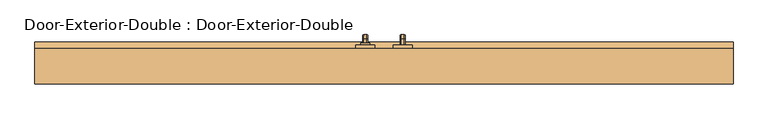
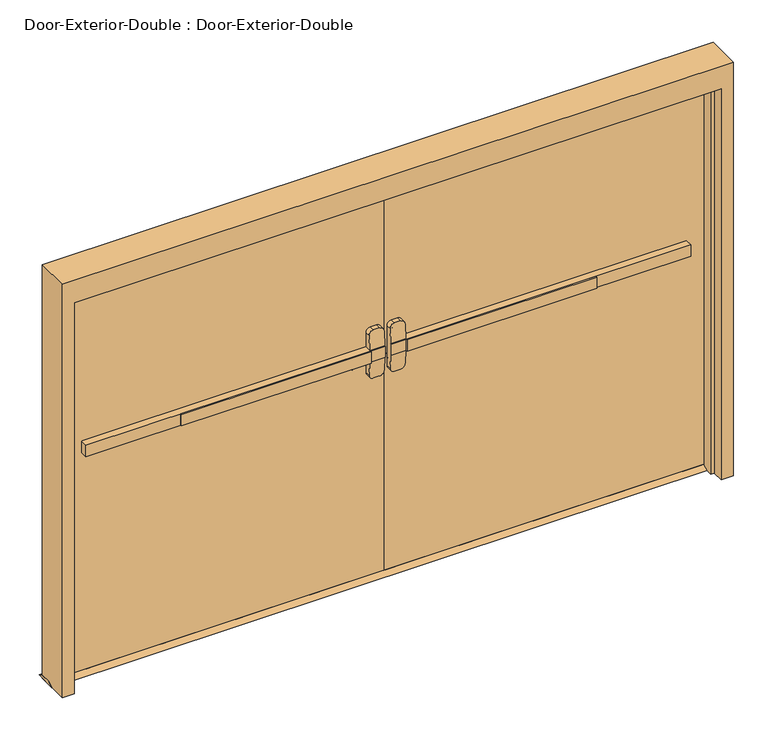
"""IFC4 building model written with IfcOpenShell, lengths in millimetres: door geometry, Door-Exterior-Double : Door-Exterior-Double."""

from ifc_helpers import new_model, si_unit, point, frame, frame_2d, origin, place, context, project, spatial, polyline, circle_curve, ellipse_curve, trimmed, segment, composite_curve, outline, extrude, faceted_brep, source, transform, mapped, element, save
from ifc_brep_helpers import plane_surface, cylinder_surface, revolved_surface, advanced_brep


def door_exterior_double_door_exterior_double_ceddc7a2(model_context):
    return source(origin(), model_context, "Body", "SolidModel", [
        extrude(outline(polyline([(-880.5333333, 0.0), (-880.5333333, 6.35), (-76.2, 6.35), (-76.2, 0.0), (-880.5333333, 0.0)])), frame((0.0, 0.0, 990.6), z_axis=(0.0, 0.0, 1.0), x_axis=(1.0, 0.0, 0.0)), (0.0, 0.0, 1.0), 50.8),
        advanced_brep(
        [(-12.7, 6.35, 1041.4), (-76.2, 6.35, 1041.4), (-1282.7, 6.35, 1041.4), (-1282.7, 6.35, 990.6), (-76.2, 6.35, 990.6), (-12.7, 6.35, 990.6), (-1282.7, 38.1, 1041.4), (-76.2, 38.1, 1041.4), (-76.2, 38.1, 1104.9), (-57.15, 38.1, 1123.95), (-31.75, 38.1, 1123.95), (-12.7, 38.1, 1104.9), (-12.7, 38.1, 927.1), (-31.75, 38.1, 908.05), (-57.15, 38.1, 908.05), (-76.2, 38.1, 927.1), (-76.2, 38.1, 990.6), (-1282.7, 38.1, 990.6), (-12.7, 9.5252467, 1041.4), (-76.2, 9.5252467, 1041.4), (-12.7, 9.5252467, 990.6), (-12.7, 14.5354269, 927.1), (-12.7, 14.5354269, 1104.9), (-76.2, 9.5252467, 990.6), (-76.2, 14.5354269, 1104.9), (-76.2, 14.5354269, 927.1), (-57.15, 16.038481, 1123.95), (-31.75, 16.038481, 1123.95), (-31.75, 16.038481, 908.05), (-57.15, 16.038481, 908.05)],
        [
            (0, 1),
            (1, 2),
            (2, 3),
            (3, 4),
            (4, 5),
            (5, 0),
            (6, 7),
            (7, 8),
            (8, 9, circle_curve(frame((-57.15, 38.1, 1104.9), z_axis=(0.0, 1.0, 0.0), x_axis=(-1.0, 0.0, 0.0)), 19.05)),
            (9, 10),
            (10, 11, circle_curve(frame((-31.75, 38.1, 1104.9), z_axis=(0.0, 1.0, 0.0), x_axis=(-1.0, 0.0, 0.0)), 19.05)),
            (11, 12),
            (12, 13, circle_curve(frame((-31.75, 38.1, 927.1), z_axis=(0.0, 1.0, 0.0), x_axis=(-1.0, 0.0, 0.0)), 19.05)),
            (13, 14),
            (14, 15, circle_curve(frame((-57.15, 38.1, 927.1), z_axis=(0.0, 1.0, 0.0), x_axis=(-1.0, 0.0, 0.0)), 19.05)),
            (15, 16),
            (16, 17),
            (17, 6),
            (0, 18),
            (18, 19),
            (19, 7),
            (6, 2),
            (5, 20),
            (20, 21),
            (21, 12),
            (11, 22),
            (22, 18),
            (16, 23),
            (23, 20),
            (3, 17),
            (19, 24),
            (24, 8),
            (15, 25),
            (25, 23),
            (9, 26),
            (26, 27),
            (27, 10),
            (13, 28),
            (28, 29),
            (29, 14),
            (29, 25, ellipse_curve(frame((-57.15, 14.5354269, 927.1), z_axis=(0.0, 0.9969018152893365, 0.07865602756830282), x_axis=(0.0, -0.07865602756830208, 0.9969018152893365)), 19.1092038, 19.05)),
            (24, 26, ellipse_curve(frame((-57.15, 14.5354269, 1104.9), z_axis=(0.0, 0.9969018152893376, -0.07865602756828934), x_axis=(0.0, -0.078656027568288, -0.9969018152893377)), 19.1092038, 19.05)),
            (27, 22, ellipse_curve(frame((-31.75, 14.5354269, 1104.9), z_axis=(0.0, 0.9969018152893376, -0.07865602756828934), x_axis=(0.0, -0.078656027568288, -0.9969018152893377)), 19.1092038, 19.05)),
            (21, 28, ellipse_curve(frame((-31.75, 14.5354269, 927.1), z_axis=(0.0, 0.9969018152893365, 0.07865602756830282), x_axis=(0.0, -0.07865602756830208, 0.9969018152893365)), 19.1092038, 19.05)),
        ],
        [
            plane_surface(frame((-12.7, 6.35, 1041.4), z_axis=(0.0, -1.0, 0.0), x_axis=(1.0, 0.0, 0.0))),
            plane_surface(frame((-12.7, 38.1, 1041.4), z_axis=(0.0, 1.0, 0.0), x_axis=(-1.0, 0.0, 0.0))),
            plane_surface(frame((-1282.7, 6.35, 1041.4), z_axis=(0.0, 0.0, 1.0), x_axis=(0.0, 1.0, 0.0))),
            plane_surface(frame((-12.7, 6.35, 1041.4), z_axis=(1.0, 0.0, 0.0), x_axis=(0.0, 1.0, 0.0))),
            plane_surface(frame((-12.7, 6.35, 990.6), z_axis=(0.0, 0.0, -1.0), x_axis=(0.0, 1.0, 0.0))),
            plane_surface(frame((-1282.7, 6.35, 990.6), z_axis=(-1.0, 0.0, 0.0), x_axis=(0.0, 1.0, 0.0))),
            plane_surface(frame((-76.2, 9.5252467, 927.1), z_axis=(-1.0, 0.0, 0.0), x_axis=(0.0, 1.0, 0.0))),
            plane_surface(frame((-57.15, 9.5252467, 1123.95), z_axis=(0.0, 0.0, 1.0), x_axis=(0.0, 1.0, 0.0))),
            plane_surface(frame((-31.75, 9.5252467, 908.05), z_axis=(0.0, 0.0, -1.0), x_axis=(0.0, 1.0, 0.0))),
            cylinder_surface(frame((-57.15, 38.1, 927.1), z_axis=(0.0, -1.0, 0.0), x_axis=(-1.0, 0.0, 0.0)), 19.05),
            cylinder_surface(frame((-57.15, 38.1, 1104.9), z_axis=(0.0, -1.0, 0.0), x_axis=(-1.0, 0.0, 0.0)), 19.05),
            cylinder_surface(frame((-31.75, 38.1, 1104.9), z_axis=(0.0, -1.0, 0.0), x_axis=(-1.0, 0.0, 0.0)), 19.05),
            cylinder_surface(frame((-31.75, 38.1, 927.1), z_axis=(0.0, -1.0, 0.0), x_axis=(-1.0, 0.0, 0.0)), 19.05),
            plane_surface(frame((-76.2, 9.5252467, 1041.4), z_axis=(0.0, -0.9969018152893376, 0.07865602756828934), x_axis=(1.0, 0.0, 0.0))),
            plane_surface(frame((-76.2, 16.038481, 908.05), z_axis=(0.0, -0.9969018152893365, -0.07865602756830282), x_axis=(1.0, 0.0, 0.0))),
        ],
        [
            (0, [[1, 2, 3, 4, 5, 6]]),
            (1, [[7, 8, 9, 10, 11, 12, 13, 14, 15, 16, 17, 18]]),
            (2, [[-2, -1, 19, 20, 21, -7, 22]]),
            (3, [[23, 24, 25, -12, 26, 27, -19, -6]]),
            (4, [[-17, 28, 29, -23, -5, -4, 30]]),
            (5, [[-22, -18, -30, -3]]),
            (6, [[-21, 31, 32, -8]]),
            (6, [[33, 34, -28, -16]]),
            (7, [[35, 36, 37, -10]]),
            (8, [[38, 39, 40, -14]]),
            (9, [[-40, 41, -33, -15]]),
            (10, [[-32, 42, -35, -9]]),
            (11, [[-37, 43, -26, -11]]),
            (12, [[-25, 44, -38, -13]]),
            (13, [[-27, -43, -36, -42, -31, -20]]),
            (14, [[-29, -34, -41, -39, -44, -24]]),
        ],
    ),
        extrude(outline(polyline([(82.55, 12.7), (107.95, 0.0), (12.7, 0.0), (38.1, 12.7), (82.55, 12.7)])), frame((-1422.4, 0.0, 0.0), z_axis=(1.0, 0.0, 0.0), x_axis=(0.0, 1.0, 0.0)), (0.0, 0.0, 1.0), 2844.8),
        extrude(outline(polyline([(880.5333333, 0.0), (76.2, 0.0), (76.2, 6.35), (880.5333333, 6.35), (880.5333333, 0.0)])), frame((0.0, 0.0, 990.6), z_axis=(0.0, 0.0, 1.0), x_axis=(1.0, 0.0, 0.0)), (0.0, 0.0, 1.0), 50.8),
        advanced_brep(
        [(12.7, 6.35, 1041.4), (12.7, 6.35, 990.6), (76.2, 6.35, 990.6), (1282.7, 6.35, 990.6), (1282.7, 6.35, 1041.4), (76.2, 6.35, 1041.4), (1282.7, 38.1, 1041.4), (1282.7, 38.1, 990.6), (76.2, 38.1, 990.6), (76.2, 38.1, 927.1), (57.15, 38.1, 908.05), (31.75, 38.1, 908.05), (12.7, 38.1, 927.1), (12.7, 38.1, 1104.9), (31.75, 38.1, 1123.95), (57.15, 38.1, 1123.95), (76.2, 38.1, 1104.9), (76.2, 38.1, 1041.4), (76.2, 9.5252467, 1041.4), (12.7, 9.5252467, 1041.4), (12.7, 14.5354269, 1104.9), (12.7, 14.5354269, 927.1), (12.7, 9.5252467, 990.6), (76.2, 9.5252467, 990.6), (76.2, 14.5354269, 927.1), (76.2, 14.5354269, 1104.9), (31.75, 16.038481, 1123.95), (57.15, 16.038481, 1123.95), (57.15, 16.038481, 908.05), (31.75, 16.038481, 908.05)],
        [
            (0, 1),
            (1, 2),
            (2, 3),
            (3, 4),
            (4, 5),
            (5, 0),
            (6, 7),
            (7, 8),
            (8, 9),
            (9, 10, circle_curve(frame((57.15, 38.1, 927.1), z_axis=(0.0, 1.0, 0.0), x_axis=(1.0, 0.0, 0.0)), 19.05)),
            (10, 11),
            (11, 12, circle_curve(frame((31.75, 38.1, 927.1), z_axis=(0.0, 1.0, 0.0), x_axis=(1.0, 0.0, 0.0)), 19.05)),
            (12, 13),
            (13, 14, circle_curve(frame((31.75, 38.1, 1104.9), z_axis=(0.0, 1.0, 0.0), x_axis=(1.0, 0.0, 0.0)), 19.05)),
            (14, 15),
            (15, 16, circle_curve(frame((57.15, 38.1, 1104.9), z_axis=(0.0, 1.0, 0.0), x_axis=(1.0, 0.0, 0.0)), 19.05)),
            (16, 17),
            (17, 6),
            (4, 6),
            (17, 18),
            (18, 19),
            (19, 0),
            (19, 20),
            (20, 13),
            (12, 21),
            (21, 22),
            (22, 1),
            (7, 3),
            (22, 23),
            (23, 8),
            (23, 24),
            (24, 9),
            (16, 25),
            (25, 18),
            (14, 26),
            (26, 27),
            (27, 15),
            (10, 28),
            (28, 29),
            (29, 11),
            (24, 28, ellipse_curve(frame((57.15, 14.5354269, 927.1), z_axis=(0.0, 0.9969018152893365, 0.07865602756830282), x_axis=(0.0, -0.07865602756830208, 0.9969018152893365)), 19.1092038, 19.05)),
            (27, 25, ellipse_curve(frame((57.15, 14.5354269, 1104.9), z_axis=(0.0, 0.9969018152893376, -0.07865602756828934), x_axis=(0.0, -0.078656027568288, -0.9969018152893377)), 19.1092038, 19.05)),
            (20, 26, ellipse_curve(frame((31.75, 14.5354269, 1104.9), z_axis=(0.0, 0.9969018152893376, -0.07865602756828934), x_axis=(0.0, -0.078656027568288, -0.9969018152893377)), 19.1092038, 19.05)),
            (29, 21, ellipse_curve(frame((31.75, 14.5354269, 927.1), z_axis=(0.0, 0.9969018152893365, 0.07865602756830282), x_axis=(0.0, -0.07865602756830208, 0.9969018152893365)), 19.1092038, 19.05)),
        ],
        [
            plane_surface(frame((12.7, 6.35, 1041.4), z_axis=(0.0, -1.0, 0.0), x_axis=(-1.0, 0.0, 0.0))),
            plane_surface(frame((12.7, 38.1, 1041.4), z_axis=(0.0, 1.0, 0.0), x_axis=(1.0, 0.0, 0.0))),
            plane_surface(frame((1282.7, 6.35, 1041.4), z_axis=(0.0, 0.0, 1.0), x_axis=(0.0, 1.0, 0.0))),
            plane_surface(frame((12.7, 6.35, 1041.4), z_axis=(-1.0, 0.0, 0.0), x_axis=(0.0, 1.0, 0.0))),
            plane_surface(frame((12.7, 6.35, 990.6), z_axis=(0.0, 0.0, -1.0), x_axis=(0.0, 1.0, 0.0))),
            plane_surface(frame((1282.7, 6.35, 990.6), z_axis=(1.0, 0.0, 0.0), x_axis=(0.0, 1.0, 0.0))),
            plane_surface(frame((76.2, 9.5252467, 927.1), z_axis=(1.0, 0.0, 0.0), x_axis=(0.0, 1.0, 0.0))),
            plane_surface(frame((57.15, 9.5252467, 1123.95), z_axis=(0.0, 0.0, 1.0), x_axis=(0.0, 1.0, 0.0))),
            plane_surface(frame((31.75, 9.5252467, 908.05), z_axis=(0.0, 0.0, -1.0), x_axis=(0.0, 1.0, 0.0))),
            cylinder_surface(frame((57.15, 38.1, 927.1), z_axis=(0.0, -1.0, 0.0), x_axis=(1.0, 0.0, 0.0)), 19.05),
            cylinder_surface(frame((57.15, 38.1, 1104.9), z_axis=(0.0, -1.0, 0.0), x_axis=(1.0, 0.0, 0.0)), 19.05),
            cylinder_surface(frame((31.75, 38.1, 1104.9), z_axis=(0.0, -1.0, 0.0), x_axis=(1.0, 0.0, 0.0)), 19.05),
            cylinder_surface(frame((31.75, 38.1, 927.1), z_axis=(0.0, -1.0, 0.0), x_axis=(1.0, 0.0, 0.0)), 19.05),
            plane_surface(frame((76.2, 9.5252467, 1041.4), z_axis=(0.0, -0.9969018152893376, 0.07865602756828934), x_axis=(-1.0, 0.0, 0.0))),
            plane_surface(frame((76.2, 16.038481, 908.05), z_axis=(0.0, -0.9969018152893365, -0.07865602756830282), x_axis=(-1.0, 0.0, 0.0))),
        ],
        [
            (0, [[1, 2, 3, 4, 5, 6]]),
            (1, [[7, 8, 9, 10, 11, 12, 13, 14, 15, 16, 17, 18]]),
            (2, [[19, -18, 20, 21, 22, -6, -5]]),
            (3, [[-1, -22, 23, 24, -13, 25, 26, 27]]),
            (4, [[28, -3, -2, -27, 29, 30, -8]]),
            (5, [[-4, -28, -7, -19]]),
            (6, [[-9, -30, 31, 32]]),
            (6, [[-17, 33, 34, -20]]),
            (7, [[-15, 35, 36, 37]]),
            (8, [[-11, 38, 39, 40]]),
            (9, [[-10, -32, 41, -38]]),
            (10, [[-16, -37, 42, -33]]),
            (11, [[-14, -24, 43, -35]]),
            (12, [[-12, -40, 44, -25]]),
            (13, [[-21, -34, -42, -36, -43, -23]]),
            (14, [[-26, -44, -39, -41, -31, -29]]),
        ],
    ),
        advanced_brep(
        [(66.2, 95.25, 1017.190625), (66.2, 95.25, 1014.809375), (69.771875, 95.25, 1011.2375), (82.6284594, 95.25, 1011.2375), (86.2, 95.25, 1014.8090406), (86.2, 95.25, 1017.190625), (82.628125, 95.25, 1020.7625), (69.771875, 95.25, 1020.7625), (66.2, 95.25, 887.809375), (69.771875, 95.25, 884.2375), (82.628125, 95.25, 884.2375), (86.2, 95.25, 887.809375), (86.2, 95.25, 890.1909594), (82.6284594, 95.25, 893.7625), (69.771875, 95.25, 893.7625), (66.2, 95.25, 890.190625), (66.2, 120.65, 1017.190625), (66.2, 134.540625, 1003.3), (66.2, 134.540625, 901.7), (66.2, 120.65, 887.809375), (66.2, 120.65, 890.190625), (66.2, 132.159375, 901.7), (66.2, 132.159375, 1003.3), (66.2, 120.65, 1014.809375), (69.771875, 120.65, 1011.2375), (82.6284594, 120.65, 1011.2375), (86.2, 120.65, 1014.8090406), (86.2, 132.1590406, 1003.3), (86.2, 132.1590406, 901.7), (86.2, 120.65, 890.1909594), (86.2, 120.65, 887.809375), (86.2, 134.540625, 901.7), (86.2, 134.540625, 1003.3), (86.2, 120.65, 1017.190625), (82.628125, 120.65, 1020.7625), (69.771875, 120.65, 1020.7625), (69.771875, 128.5875, 1003.3), (82.6284594, 128.5875, 1003.3), (82.628125, 138.1125, 1003.3), (69.771875, 138.1125, 1003.3), (69.771875, 128.5875, 901.7), (82.6284594, 128.5875, 901.7), (82.628125, 138.1125, 901.7), (69.771875, 138.1125, 901.7), (69.771875, 120.65, 893.7625), (82.6284594, 120.65, 893.7625), (82.628125, 120.65, 884.2375), (69.771875, 120.65, 884.2375)],
        [
            (0, 1),
            (1, 2, circle_curve(frame((69.771875, 95.25, 1014.809375), z_axis=(0.0, -1.0, 0.0), x_axis=(0.0, 0.0, 1.0)), 3.571875)),
            (2, 3),
            (3, 4, circle_curve(frame((82.6284594, 95.25, 1014.8090406), z_axis=(0.0, -1.0, 0.0), x_axis=(0.0, 0.0, 1.0)), 3.5715406)),
            (4, 5),
            (5, 6, circle_curve(frame((82.628125, 95.25, 1017.190625), z_axis=(0.0, -1.0, 0.0), x_axis=(0.0, 0.0, 1.0)), 3.571875)),
            (6, 7),
            (7, 0, circle_curve(frame((69.771875, 95.25, 1017.190625), z_axis=(0.0, -1.0, 0.0), x_axis=(0.0, 0.0, 1.0)), 3.571875)),
            (8, 9, circle_curve(frame((69.771875, 95.25, 887.809375), z_axis=(0.0, -1.0, 0.0), x_axis=(0.0, 0.0, -1.0)), 3.571875)),
            (9, 10),
            (10, 11, circle_curve(frame((82.628125, 95.25, 887.809375), z_axis=(0.0, -1.0, 0.0), x_axis=(0.0, 0.0, -1.0)), 3.571875)),
            (11, 12),
            (12, 13, circle_curve(frame((82.6284594, 95.25, 890.1909594), z_axis=(0.0, -1.0, 0.0), x_axis=(0.0, 0.0, -1.0)), 3.5715406)),
            (13, 14),
            (14, 15, circle_curve(frame((69.771875, 95.25, 890.190625), z_axis=(0.0, -1.0, 0.0), x_axis=(0.0, 0.0, -1.0)), 3.571875)),
            (15, 8),
            (0, 16),
            (16, 17, circle_curve(frame((66.2, 120.65, 1003.3), z_axis=(-1.0, 0.0, 0.0), x_axis=(0.0, 0.0, 1.0)), 13.890625)),
            (17, 18),
            (18, 19, circle_curve(frame((66.2, 120.65, 901.7), z_axis=(-1.0, 0.0, 0.0), x_axis=(0.0, 1.0, 0.0)), 13.890625)),
            (19, 8),
            (15, 20),
            (20, 21, circle_curve(frame((66.2, 120.65, 901.7), z_axis=(1.0, 0.0, 0.0), x_axis=(0.0, 1.0, 0.0)), 11.509375)),
            (21, 22),
            (22, 23, circle_curve(frame((66.2, 120.65, 1003.3), z_axis=(1.0, 0.0, 0.0), x_axis=(0.0, 0.0, 1.0)), 11.509375)),
            (23, 1),
            (23, 24, circle_curve(frame((69.771875, 120.65, 1014.809375), z_axis=(0.0, -1.0, 0.0), x_axis=(0.0, 0.0, 1.0)), 3.571875)),
            (24, 2),
            (24, 25),
            (25, 3),
            (25, 26, circle_curve(frame((82.6284594, 120.65, 1014.8090406), z_axis=(0.0, -1.0, 0.0), x_axis=(0.0, 0.0, 1.0)), 3.5715406)),
            (26, 4),
            (26, 27, circle_curve(frame((86.2, 120.65, 1003.3), z_axis=(-1.0, 0.0, 0.0), x_axis=(0.0, 0.0, 1.0)), 11.5090406)),
            (27, 28),
            (28, 29, circle_curve(frame((86.2, 120.65, 901.7), z_axis=(-1.0, 0.0, 0.0), x_axis=(0.0, 1.0, 0.0)), 11.5090406)),
            (29, 12),
            (11, 30),
            (30, 31, circle_curve(frame((86.2, 120.65, 901.7), z_axis=(1.0, 0.0, 0.0), x_axis=(0.0, 1.0, 0.0)), 13.890625)),
            (31, 32),
            (32, 33, circle_curve(frame((86.2, 120.65, 1003.3), z_axis=(1.0, 0.0, 0.0), x_axis=(0.0, 0.0, 1.0)), 13.890625)),
            (33, 5),
            (33, 34, circle_curve(frame((82.628125, 120.65, 1017.190625), z_axis=(0.0, -1.0, 0.0), x_axis=(0.0, 0.0, 1.0)), 3.571875)),
            (34, 6),
            (34, 35),
            (35, 7),
            (35, 16, circle_curve(frame((69.771875, 120.65, 1017.190625), z_axis=(0.0, -1.0, 0.0), x_axis=(0.0, 0.0, 1.0)), 3.571875)),
            (36, 24, circle_curve(frame((69.771875, 120.65, 1003.3), z_axis=(1.0, 0.0, 0.0), x_axis=(0.0, 0.0, 1.0)), 7.9375)),
            (22, 36, circle_curve(frame((69.771875, 132.159375, 1003.3), z_axis=(0.0, 0.0, 1.0), x_axis=(0.0, 1.0, 0.0)), 3.571875)),
            (37, 25, circle_curve(frame((82.6284594, 120.65, 1003.3), z_axis=(1.0, 0.0, 0.0), x_axis=(0.0, 0.0, 1.0)), 7.9375)),
            (36, 37),
            (37, 27, circle_curve(frame((82.6284594, 132.1590406, 1003.3), z_axis=(0.0, 0.0, 1.0), x_axis=(0.0, 1.0, 0.0)), 3.5715406)),
            (38, 34, circle_curve(frame((82.628125, 120.65, 1003.3), z_axis=(1.0, 0.0, 0.0), x_axis=(0.0, 0.0, 1.0)), 17.4625)),
            (32, 38, circle_curve(frame((82.628125, 134.540625, 1003.3), z_axis=(0.0, 0.0, 1.0), x_axis=(0.0, 1.0, 0.0)), 3.571875)),
            (39, 35, circle_curve(frame((69.771875, 120.65, 1003.3), z_axis=(1.0, 0.0, 0.0), x_axis=(0.0, 0.0, 1.0)), 17.4625)),
            (38, 39),
            (39, 17, circle_curve(frame((69.771875, 134.540625, 1003.3), z_axis=(0.0, 0.0, 1.0), x_axis=(0.0, 1.0, 0.0)), 3.571875)),
            (21, 40, circle_curve(frame((69.771875, 132.159375, 901.7), z_axis=(0.0, 0.0, 1.0), x_axis=(0.0, 1.0, 0.0)), 3.571875)),
            (40, 36),
            (40, 41),
            (41, 37),
            (41, 28, circle_curve(frame((82.6284594, 132.1590406, 901.7), z_axis=(0.0, 0.0, 1.0), x_axis=(0.0, 1.0, 0.0)), 3.5715406)),
            (31, 42, circle_curve(frame((82.628125, 134.540625, 901.7), z_axis=(0.0, 0.0, 1.0), x_axis=(0.0, 1.0, 0.0)), 3.571875)),
            (42, 38),
            (42, 43),
            (43, 39),
            (43, 18, circle_curve(frame((69.771875, 134.540625, 901.7), z_axis=(0.0, 0.0, 1.0), x_axis=(0.0, 1.0, 0.0)), 3.571875)),
            (44, 40, circle_curve(frame((69.771875, 120.65, 901.7), z_axis=(1.0, 0.0, 0.0), x_axis=(0.0, 1.0, 0.0)), 7.9375)),
            (20, 44, circle_curve(frame((69.771875, 120.65, 890.190625), z_axis=(0.0, 1.0, 0.0), x_axis=(0.0, 0.0, -1.0)), 3.571875)),
            (45, 41, circle_curve(frame((82.6284594, 120.65, 901.7), z_axis=(1.0, 0.0, 0.0), x_axis=(0.0, 1.0, 0.0)), 7.9375)),
            (44, 45),
            (45, 29, circle_curve(frame((82.6284594, 120.65, 890.1909594), z_axis=(0.0, 1.0, 0.0), x_axis=(0.0, 0.0, -1.0)), 3.5715406)),
            (46, 42, circle_curve(frame((82.628125, 120.65, 901.7), z_axis=(1.0, 0.0, 0.0), x_axis=(0.0, 1.0, 0.0)), 17.4625)),
            (30, 46, circle_curve(frame((82.628125, 120.65, 887.809375), z_axis=(0.0, 1.0, 0.0), x_axis=(0.0, 0.0, -1.0)), 3.571875)),
            (47, 43, circle_curve(frame((69.771875, 120.65, 901.7), z_axis=(1.0, 0.0, 0.0), x_axis=(0.0, 1.0, 0.0)), 17.4625)),
            (46, 47),
            (47, 19, circle_curve(frame((69.771875, 120.65, 887.809375), z_axis=(0.0, 1.0, 0.0), x_axis=(0.0, 0.0, -1.0)), 3.571875)),
            (14, 44),
            (13, 45),
            (10, 46),
            (9, 47),
        ],
        [
            plane_surface(frame((76.2, 95.25, 1016.0), z_axis=(0.0, -1.0, 0.0), x_axis=(1.0, 0.0, 0.0))),
            plane_surface(frame((76.2, 95.25, 889.0), z_axis=(0.0, -1.0, 0.0), x_axis=(1.0, 0.0, 0.0))),
            plane_surface(frame((66.2, 95.25, 1017.190625), z_axis=(-1.0, 0.0, 0.0), x_axis=(0.0, 1.0, 0.0))),
            cylinder_surface(frame((69.771875, 95.25, 1014.809375), z_axis=(0.0, -1.0, 0.0), x_axis=(0.0, 0.0, 1.0)), 3.571875),
            plane_surface(frame((69.771875, 95.25, 1011.2375), z_axis=(0.0, 0.0, -1.0), x_axis=(0.0, 1.0, 0.0))),
            cylinder_surface(frame((82.6284594, 95.25, 1014.8090406), z_axis=(0.0, -1.0, 0.0), x_axis=(0.0, 0.0, 1.0)), 3.5715406),
            plane_surface(frame((86.2, 95.25, 1014.8090406), z_axis=(1.0, 0.0, 0.0), x_axis=(0.0, 1.0, 0.0))),
            cylinder_surface(frame((82.628125, 95.25, 1017.190625), z_axis=(0.0, -1.0, 0.0), x_axis=(0.0, 0.0, 1.0)), 3.571875),
            plane_surface(frame((82.628125, 95.25, 1020.7625), z_axis=(0.0, 0.0, 1.0), x_axis=(0.0, 1.0, 0.0))),
            cylinder_surface(frame((69.771875, 95.25, 1017.190625), z_axis=(0.0, -1.0, 0.0), x_axis=(0.0, 0.0, 1.0)), 3.571875),
            revolved_surface(trimmed(ellipse_curve(frame((69.771875, 120.65, 1014.809375), z_axis=(0.0, -1.0, 0.0), x_axis=(0.0, 0.0, 1.0)), 3.571875, 3.571875), [point((66.2, 120.65, 1014.809375))], [point((69.771875, 120.65, 1011.2375))], True, "CARTESIAN"), (76.2, 120.65, 1003.3), (-1.0, 0.0, 0.0)),
            revolved_surface(polyline([(69.771875, 120.65, 1011.2375), (82.6284594, 120.65, 1011.2375)]), (76.2, 120.65, 1003.3), (-1.0, 0.0, 0.0)),
            revolved_surface(trimmed(ellipse_curve(frame((82.6284594, 120.65, 1014.8090406), z_axis=(0.0, -1.0, 0.0), x_axis=(0.0, 0.0, 1.0)), 3.5715406, 3.5715406), [point((82.6284594, 120.65, 1011.2375))], [point((86.2, 120.65, 1014.8090406))], True, "CARTESIAN"), (76.2, 120.65, 1003.3), (-1.0, 0.0, 0.0)),
            revolved_surface(trimmed(ellipse_curve(frame((82.628125, 120.65, 1017.190625), z_axis=(0.0, -1.0, 0.0), x_axis=(0.0, 0.0, 1.0)), 3.571875, 3.571875), [point((86.2, 120.65, 1017.190625))], [point((82.628125, 120.65, 1020.7625))], True, "CARTESIAN"), (76.2, 120.65, 1003.3), (-1.0, 0.0, 0.0)),
            cylinder_surface(frame((76.2, 120.65, 1003.3), z_axis=(-1.0, 0.0, 0.0), x_axis=(0.0, 0.0, 1.0)), 17.4625),
            revolved_surface(trimmed(ellipse_curve(frame((69.771875, 120.65, 1017.190625), z_axis=(0.0, -1.0, 0.0), x_axis=(0.0, 0.0, 1.0)), 3.571875, 3.571875), [point((69.771875, 120.65, 1020.7625))], [point((66.2, 120.65, 1017.190625))], True, "CARTESIAN"), (76.2, 120.65, 1003.3), (-1.0, 0.0, 0.0)),
            cylinder_surface(frame((69.771875, 132.159375, 1003.3), z_axis=(0.0, 0.0, 1.0), x_axis=(0.0, 1.0, 0.0)), 3.571875),
            plane_surface(frame((69.771875, 128.5875, 1003.3), z_axis=(0.0, -1.0, 0.0), x_axis=(0.0, 0.0, -1.0))),
            cylinder_surface(frame((82.6284594, 132.1590406, 1003.3), z_axis=(0.0, 0.0, 1.0), x_axis=(0.0, 1.0, 0.0)), 3.5715406),
            cylinder_surface(frame((82.628125, 134.540625, 1003.3), z_axis=(0.0, 0.0, 1.0), x_axis=(0.0, 1.0, 0.0)), 3.571875),
            plane_surface(frame((82.628125, 138.1125, 1003.3), z_axis=(0.0, 1.0, 0.0), x_axis=(0.0, 0.0, -1.0))),
            cylinder_surface(frame((69.771875, 134.540625, 1003.3), z_axis=(0.0, 0.0, 1.0), x_axis=(0.0, 1.0, 0.0)), 3.571875),
            revolved_surface(trimmed(ellipse_curve(frame((69.771875, 132.159375, 901.7), z_axis=(0.0, 0.0, 1.0), x_axis=(0.0, 1.0, 0.0)), 3.571875, 3.571875), [point((66.2, 132.159375, 901.7))], [point((69.771875, 128.5875, 901.7))], True, "CARTESIAN"), (76.2, 120.65, 901.7), (-1.0, 0.0, 0.0)),
            revolved_surface(polyline([(69.771875, 128.5875, 901.7), (82.6284594, 128.5875, 901.7)]), (76.2, 120.65, 901.7), (-1.0, 0.0, 0.0)),
            revolved_surface(trimmed(ellipse_curve(frame((82.6284594, 132.1590406, 901.7), z_axis=(0.0, 0.0, 1.0), x_axis=(0.0, 1.0, 0.0)), 3.5715406, 3.5715406), [point((82.6284594, 128.5875, 901.7))], [point((86.2, 132.1590406, 901.7))], True, "CARTESIAN"), (76.2, 120.65, 901.7), (-1.0, 0.0, 0.0)),
            revolved_surface(trimmed(ellipse_curve(frame((82.628125, 134.540625, 901.7), z_axis=(0.0, 0.0, 1.0), x_axis=(0.0, 1.0, 0.0)), 3.571875, 3.571875), [point((86.2, 134.540625, 901.7))], [point((82.628125, 138.1125, 901.7))], True, "CARTESIAN"), (76.2, 120.65, 901.7), (-1.0, 0.0, 0.0)),
            cylinder_surface(frame((76.2, 120.65, 901.7), z_axis=(-1.0, 0.0, 0.0), x_axis=(0.0, 1.0, 0.0)), 17.4625),
            revolved_surface(trimmed(ellipse_curve(frame((69.771875, 134.540625, 901.7), z_axis=(0.0, 0.0, 1.0), x_axis=(0.0, 1.0, 0.0)), 3.571875, 3.571875), [point((69.771875, 138.1125, 901.7))], [point((66.2, 134.540625, 901.7))], True, "CARTESIAN"), (76.2, 120.65, 901.7), (-1.0, 0.0, 0.0)),
            cylinder_surface(frame((69.771875, 120.65, 890.190625), z_axis=(0.0, 1.0, 0.0), x_axis=(0.0, 0.0, -1.0)), 3.571875),
            plane_surface(frame((69.771875, 120.65, 893.7625), z_axis=(0.0, 0.0, 1.0), x_axis=(0.0, -1.0, 0.0))),
            cylinder_surface(frame((82.6284594, 120.65, 890.1909594), z_axis=(0.0, 1.0, 0.0), x_axis=(0.0, 0.0, -1.0)), 3.5715406),
            cylinder_surface(frame((82.628125, 120.65, 887.809375), z_axis=(0.0, 1.0, 0.0), x_axis=(0.0, 0.0, -1.0)), 3.571875),
            plane_surface(frame((82.628125, 120.65, 884.2375), z_axis=(0.0, 0.0, -1.0), x_axis=(0.0, -1.0, 0.0))),
            cylinder_surface(frame((69.771875, 120.65, 887.809375), z_axis=(0.0, 1.0, 0.0), x_axis=(0.0, 0.0, -1.0)), 3.571875),
        ],
        [
            (0, [[1, 2, 3, 4, 5, 6, 7, 8]]),
            (1, [[9, 10, 11, 12, 13, 14, 15, 16]]),
            (2, [[-1, 17, 18, 19, 20, 21, -16, 22, 23, 24, 25, 26]]),
            (3, [[-2, -26, 27, 28]]),
            (4, [[-3, -28, 29, 30]]),
            (5, [[-4, -30, 31, 32]]),
            (6, [[-5, -32, 33, 34, 35, 36, -12, 37, 38, 39, 40, 41]]),
            (7, [[-6, -41, 42, 43]]),
            (8, [[-7, -43, 44, 45]]),
            (9, [[-8, -45, 46, -17]]),
            (10, [[47, -27, -25, 48]]),
            (11, [[49, -29, -47, 50]]),
            (12, [[-33, -31, -49, 51]]),
            (13, [[52, -42, -40, 53]]),
            (14, [[54, -44, -52, 55]]),
            (15, [[-18, -46, -54, 56]]),
            (16, [[-48, -24, 57, 58]]),
            (17, [[-50, -58, 59, 60]]),
            (18, [[-51, -60, 61, -34]]),
            (19, [[-53, -39, 62, 63]]),
            (20, [[-55, -63, 64, 65]]),
            (21, [[-56, -65, 66, -19]]),
            (22, [[67, -57, -23, 68]]),
            (23, [[69, -59, -67, 70]]),
            (24, [[-35, -61, -69, 71]]),
            (25, [[72, -62, -38, 73]]),
            (26, [[74, -64, -72, 75]]),
            (27, [[-20, -66, -74, 76]]),
            (28, [[-68, -22, -15, 77]]),
            (29, [[-70, -77, -14, 78]]),
            (30, [[-71, -78, -13, -36]]),
            (31, [[-73, -37, -11, 79]]),
            (32, [[-75, -79, -10, 80]]),
            (33, [[-76, -80, -9, -21]]),
        ],
    ),
        extrude(outline(composite_curve([segment(trimmed(circle_curve(frame_2d((1113.0338574, 76.2)), 89.3016225), [point((1193.8, 114.3))], [point((1193.8, 38.1))], False, "CARTESIAN"), True, "CONTINUOUS"), segment(polyline([(1193.8, 38.1), (838.2, 38.1)]), True, "CONTINUOUS"), segment(trimmed(circle_curve(frame_2d((918.9661426, 76.2)), 89.3016225), [point((838.2, 38.1))], [point((838.2, 114.3))], False, "CARTESIAN"), True, "CONTINUOUS"), segment(polyline([(838.2, 114.3), (1193.8, 114.3)]), True, "CONTINUOUS")], self_intersect=False)), frame((0.0, 82.55, 0.0), z_axis=(0.0, 1.0, 0.0), x_axis=(0.0, 0.0, 1.0)), (0.0, 0.0, 1.0), 12.7),
        advanced_brep(
        [(-86.2, 95.25, 1017.190625), (-86.2, 95.25, 1014.809375), (-82.628125, 95.25, 1011.2375), (-69.7715406, 95.25, 1011.2375), (-66.2, 95.25, 1014.8090406), (-66.2, 95.25, 1017.190625), (-69.771875, 95.25, 1020.7625), (-82.628125, 95.25, 1020.7625), (-86.2, 95.25, 887.809375), (-82.628125, 95.25, 884.2375), (-69.771875, 95.25, 884.2375), (-66.2, 95.25, 887.809375), (-66.2, 95.25, 890.1909594), (-69.7715406, 95.25, 893.7625), (-82.628125, 95.25, 893.7625), (-86.2, 95.25, 890.190625), (-86.2, 120.65, 1017.190625), (-86.2, 134.540625, 1003.3), (-86.2, 134.540625, 901.7), (-86.2, 120.65, 887.809375), (-86.2, 120.65, 890.190625), (-86.2, 132.159375, 901.7), (-86.2, 132.159375, 1003.3), (-86.2, 120.65, 1014.809375), (-82.628125, 120.65, 1011.2375), (-69.7715406, 120.65, 1011.2375), (-66.2, 120.65, 1014.8090406), (-66.2, 132.1590406, 1003.3), (-66.2, 132.1590406, 901.7), (-66.2, 120.65, 890.1909594), (-66.2, 120.65, 887.809375), (-66.2, 134.540625, 901.7), (-66.2, 134.540625, 1003.3), (-66.2, 120.65, 1017.190625), (-69.771875, 120.65, 1020.7625), (-82.628125, 120.65, 1020.7625), (-82.628125, 128.5875, 1003.3), (-69.7715406, 128.5875, 1003.3), (-69.771875, 138.1125, 1003.3), (-82.628125, 138.1125, 1003.3), (-82.628125, 128.5875, 901.7), (-69.7715406, 128.5875, 901.7), (-69.771875, 138.1125, 901.7), (-82.628125, 138.1125, 901.7), (-82.628125, 120.65, 893.7625), (-69.7715406, 120.65, 893.7625), (-69.771875, 120.65, 884.2375), (-82.628125, 120.65, 884.2375)],
        [
            (0, 1),
            (1, 2, circle_curve(frame((-82.628125, 95.25, 1014.809375), z_axis=(0.0, -1.0, 0.0), x_axis=(0.0, 0.0, 1.0)), 3.571875)),
            (2, 3),
            (3, 4, circle_curve(frame((-69.7715406, 95.25, 1014.8090406), z_axis=(0.0, -1.0, 0.0), x_axis=(0.0, 0.0, 1.0)), 3.5715406)),
            (4, 5),
            (5, 6, circle_curve(frame((-69.771875, 95.25, 1017.190625), z_axis=(0.0, -1.0, 0.0), x_axis=(0.0, 0.0, 1.0)), 3.571875)),
            (6, 7),
            (7, 0, circle_curve(frame((-82.628125, 95.25, 1017.190625), z_axis=(0.0, -1.0, 0.0), x_axis=(0.0, 0.0, 1.0)), 3.571875)),
            (8, 9, circle_curve(frame((-82.628125, 95.25, 887.809375), z_axis=(0.0, -1.0, 0.0), x_axis=(0.0, 0.0, -1.0)), 3.571875)),
            (9, 10),
            (10, 11, circle_curve(frame((-69.771875, 95.25, 887.809375), z_axis=(0.0, -1.0, 0.0), x_axis=(0.0, 0.0, -1.0)), 3.571875)),
            (11, 12),
            (12, 13, circle_curve(frame((-69.7715406, 95.25, 890.1909594), z_axis=(0.0, -1.0, 0.0), x_axis=(0.0, 0.0, -1.0)), 3.5715406)),
            (13, 14),
            (14, 15, circle_curve(frame((-82.628125, 95.25, 890.190625), z_axis=(0.0, -1.0, 0.0), x_axis=(0.0, 0.0, -1.0)), 3.571875)),
            (15, 8),
            (0, 16),
            (16, 17, circle_curve(frame((-86.2, 120.65, 1003.3), z_axis=(-1.0, 0.0, 0.0), x_axis=(0.0, 0.0, 1.0)), 13.890625)),
            (17, 18),
            (18, 19, circle_curve(frame((-86.2, 120.65, 901.7), z_axis=(-1.0, 0.0, 0.0), x_axis=(0.0, 1.0, 0.0)), 13.890625)),
            (19, 8),
            (15, 20),
            (20, 21, circle_curve(frame((-86.2, 120.65, 901.7), z_axis=(1.0, 0.0, 0.0), x_axis=(0.0, 1.0, 0.0)), 11.509375)),
            (21, 22),
            (22, 23, circle_curve(frame((-86.2, 120.65, 1003.3), z_axis=(1.0, 0.0, 0.0), x_axis=(0.0, 0.0, 1.0)), 11.509375)),
            (23, 1),
            (23, 24, circle_curve(frame((-82.628125, 120.65, 1014.809375), z_axis=(0.0, -1.0, 0.0), x_axis=(0.0, 0.0, 1.0)), 3.571875)),
            (24, 2),
            (24, 25),
            (25, 3),
            (25, 26, circle_curve(frame((-69.7715406, 120.65, 1014.8090406), z_axis=(0.0, -1.0, 0.0), x_axis=(0.0, 0.0, 1.0)), 3.5715406)),
            (26, 4),
            (26, 27, circle_curve(frame((-66.2, 120.65, 1003.3), z_axis=(-1.0, 0.0, 0.0), x_axis=(0.0, 0.0, 1.0)), 11.5090406)),
            (27, 28),
            (28, 29, circle_curve(frame((-66.2, 120.65, 901.7), z_axis=(-1.0, 0.0, 0.0), x_axis=(0.0, 1.0, 0.0)), 11.5090406)),
            (29, 12),
            (11, 30),
            (30, 31, circle_curve(frame((-66.2, 120.65, 901.7), z_axis=(1.0, 0.0, 0.0), x_axis=(0.0, 1.0, 0.0)), 13.890625)),
            (31, 32),
            (32, 33, circle_curve(frame((-66.2, 120.65, 1003.3), z_axis=(1.0, 0.0, 0.0), x_axis=(0.0, 0.0, 1.0)), 13.890625)),
            (33, 5),
            (33, 34, circle_curve(frame((-69.771875, 120.65, 1017.190625), z_axis=(0.0, -1.0, 0.0), x_axis=(0.0, 0.0, 1.0)), 3.571875)),
            (34, 6),
            (34, 35),
            (35, 7),
            (35, 16, circle_curve(frame((-82.628125, 120.65, 1017.190625), z_axis=(0.0, -1.0, 0.0), x_axis=(0.0, 0.0, 1.0)), 3.571875)),
            (36, 24, circle_curve(frame((-82.628125, 120.65, 1003.3), z_axis=(1.0, 0.0, 0.0), x_axis=(0.0, 0.0, 1.0)), 7.9375)),
            (22, 36, circle_curve(frame((-82.628125, 132.159375, 1003.3), z_axis=(0.0, 0.0, 1.0), x_axis=(0.0, 1.0, 0.0)), 3.571875)),
            (37, 25, circle_curve(frame((-69.7715406, 120.65, 1003.3), z_axis=(1.0, 0.0, 0.0), x_axis=(0.0, 0.0, 1.0)), 7.9375)),
            (36, 37),
            (37, 27, circle_curve(frame((-69.7715406, 132.1590406, 1003.3), z_axis=(0.0, 0.0, 1.0), x_axis=(0.0, 1.0, 0.0)), 3.5715406)),
            (38, 34, circle_curve(frame((-69.771875, 120.65, 1003.3), z_axis=(1.0, 0.0, 0.0), x_axis=(0.0, 0.0, 1.0)), 17.4625)),
            (32, 38, circle_curve(frame((-69.771875, 134.540625, 1003.3), z_axis=(0.0, 0.0, 1.0), x_axis=(0.0, 1.0, 0.0)), 3.571875)),
            (39, 35, circle_curve(frame((-82.628125, 120.65, 1003.3), z_axis=(1.0, 0.0, 0.0), x_axis=(0.0, 0.0, 1.0)), 17.4625)),
            (38, 39),
            (39, 17, circle_curve(frame((-82.628125, 134.540625, 1003.3), z_axis=(0.0, 0.0, 1.0), x_axis=(0.0, 1.0, 0.0)), 3.571875)),
            (21, 40, circle_curve(frame((-82.628125, 132.159375, 901.7), z_axis=(0.0, 0.0, 1.0), x_axis=(0.0, 1.0, 0.0)), 3.571875)),
            (40, 36),
            (40, 41),
            (41, 37),
            (41, 28, circle_curve(frame((-69.7715406, 132.1590406, 901.7), z_axis=(0.0, 0.0, 1.0), x_axis=(0.0, 1.0, 0.0)), 3.5715406)),
            (31, 42, circle_curve(frame((-69.771875, 134.540625, 901.7), z_axis=(0.0, 0.0, 1.0), x_axis=(0.0, 1.0, 0.0)), 3.571875)),
            (42, 38),
            (42, 43),
            (43, 39),
            (43, 18, circle_curve(frame((-82.628125, 134.540625, 901.7), z_axis=(0.0, 0.0, 1.0), x_axis=(0.0, 1.0, 0.0)), 3.571875)),
            (44, 40, circle_curve(frame((-82.628125, 120.65, 901.7), z_axis=(1.0, 0.0, 0.0), x_axis=(0.0, 1.0, 0.0)), 7.9375)),
            (20, 44, circle_curve(frame((-82.628125, 120.65, 890.190625), z_axis=(0.0, 1.0, 0.0), x_axis=(0.0, 0.0, -1.0)), 3.571875)),
            (45, 41, circle_curve(frame((-69.7715406, 120.65, 901.7), z_axis=(1.0, 0.0, 0.0), x_axis=(0.0, 1.0, 0.0)), 7.9375)),
            (44, 45),
            (45, 29, circle_curve(frame((-69.7715406, 120.65, 890.1909594), z_axis=(0.0, 1.0, 0.0), x_axis=(0.0, 0.0, -1.0)), 3.5715406)),
            (46, 42, circle_curve(frame((-69.771875, 120.65, 901.7), z_axis=(1.0, 0.0, 0.0), x_axis=(0.0, 1.0, 0.0)), 17.4625)),
            (30, 46, circle_curve(frame((-69.771875, 120.65, 887.809375), z_axis=(0.0, 1.0, 0.0), x_axis=(0.0, 0.0, -1.0)), 3.571875)),
            (47, 43, circle_curve(frame((-82.628125, 120.65, 901.7), z_axis=(1.0, 0.0, 0.0), x_axis=(0.0, 1.0, 0.0)), 17.4625)),
            (46, 47),
            (47, 19, circle_curve(frame((-82.628125, 120.65, 887.809375), z_axis=(0.0, 1.0, 0.0), x_axis=(0.0, 0.0, -1.0)), 3.571875)),
            (14, 44),
            (13, 45),
            (10, 46),
            (9, 47),
        ],
        [
            plane_surface(frame((-76.2, 95.25, 1016.0), z_axis=(0.0, -1.0, 0.0), x_axis=(1.0, 0.0, 0.0))),
            plane_surface(frame((-76.2, 95.25, 889.0), z_axis=(0.0, -1.0, 0.0), x_axis=(1.0, 0.0, 0.0))),
            plane_surface(frame((-86.2, 95.25, 1017.190625), z_axis=(-1.0, 0.0, 0.0), x_axis=(0.0, 1.0, 0.0))),
            cylinder_surface(frame((-82.628125, 95.25, 1014.809375), z_axis=(0.0, -1.0, 0.0), x_axis=(0.0, 0.0, 1.0)), 3.571875),
            plane_surface(frame((-82.628125, 95.25, 1011.2375), z_axis=(0.0, 0.0, -1.0), x_axis=(0.0, 1.0, 0.0))),
            cylinder_surface(frame((-69.7715406, 95.25, 1014.8090406), z_axis=(0.0, -1.0, 0.0), x_axis=(0.0, 0.0, 1.0)), 3.5715406),
            plane_surface(frame((-66.2, 95.25, 1014.8090406), z_axis=(1.0, 0.0, 0.0), x_axis=(0.0, 1.0, 0.0))),
            cylinder_surface(frame((-69.771875, 95.25, 1017.190625), z_axis=(0.0, -1.0, 0.0), x_axis=(0.0, 0.0, 1.0)), 3.571875),
            plane_surface(frame((-69.771875, 95.25, 1020.7625), z_axis=(0.0, 0.0, 1.0), x_axis=(0.0, 1.0, 0.0))),
            cylinder_surface(frame((-82.628125, 95.25, 1017.190625), z_axis=(0.0, -1.0, 0.0), x_axis=(0.0, 0.0, 1.0)), 3.571875),
            revolved_surface(trimmed(ellipse_curve(frame((-82.628125, 120.65, 1014.809375), z_axis=(0.0, -1.0, 0.0), x_axis=(0.0, 0.0, 1.0)), 3.571875, 3.571875), [point((-86.2, 120.65, 1014.809375))], [point((-82.628125, 120.65, 1011.2375))], True, "CARTESIAN"), (-76.2, 120.65, 1003.3), (-1.0, 0.0, 0.0)),
            revolved_surface(polyline([(-82.628125, 120.65, 1011.2375), (-69.7715406, 120.65, 1011.2375)]), (-76.2, 120.65, 1003.3), (-1.0, 0.0, 0.0)),
            revolved_surface(trimmed(ellipse_curve(frame((-69.7715406, 120.65, 1014.8090406), z_axis=(0.0, -1.0, 0.0), x_axis=(0.0, 0.0, 1.0)), 3.5715406, 3.5715406), [point((-69.7715406, 120.65, 1011.2375))], [point((-66.2, 120.65, 1014.8090406))], True, "CARTESIAN"), (-76.2, 120.65, 1003.3), (-1.0, 0.0, 0.0)),
            revolved_surface(trimmed(ellipse_curve(frame((-69.771875, 120.65, 1017.190625), z_axis=(0.0, -1.0, 0.0), x_axis=(0.0, 0.0, 1.0)), 3.571875, 3.571875), [point((-66.2, 120.65, 1017.190625))], [point((-69.771875, 120.65, 1020.7625))], True, "CARTESIAN"), (-76.2, 120.65, 1003.3), (-1.0, 0.0, 0.0)),
            cylinder_surface(frame((-76.2, 120.65, 1003.3), z_axis=(-1.0, 0.0, 0.0), x_axis=(0.0, 0.0, 1.0)), 17.4625),
            revolved_surface(trimmed(ellipse_curve(frame((-82.628125, 120.65, 1017.190625), z_axis=(0.0, -1.0, 0.0), x_axis=(0.0, 0.0, 1.0)), 3.571875, 3.571875), [point((-82.628125, 120.65, 1020.7625))], [point((-86.2, 120.65, 1017.190625))], True, "CARTESIAN"), (-76.2, 120.65, 1003.3), (-1.0, 0.0, 0.0)),
            cylinder_surface(frame((-82.628125, 132.159375, 1003.3), z_axis=(0.0, 0.0, 1.0), x_axis=(0.0, 1.0, 0.0)), 3.571875),
            plane_surface(frame((-82.628125, 128.5875, 1003.3), z_axis=(0.0, -1.0, 0.0), x_axis=(0.0, 0.0, -1.0))),
            cylinder_surface(frame((-69.7715406, 132.1590406, 1003.3), z_axis=(0.0, 0.0, 1.0), x_axis=(0.0, 1.0, 0.0)), 3.5715406),
            cylinder_surface(frame((-69.771875, 134.540625, 1003.3), z_axis=(0.0, 0.0, 1.0), x_axis=(0.0, 1.0, 0.0)), 3.571875),
            plane_surface(frame((-69.771875, 138.1125, 1003.3), z_axis=(0.0, 1.0, 0.0), x_axis=(0.0, 0.0, -1.0))),
            cylinder_surface(frame((-82.628125, 134.540625, 1003.3), z_axis=(0.0, 0.0, 1.0), x_axis=(0.0, 1.0, 0.0)), 3.571875),
            revolved_surface(trimmed(ellipse_curve(frame((-82.628125, 132.159375, 901.7), z_axis=(0.0, 0.0, 1.0), x_axis=(0.0, 1.0, 0.0)), 3.571875, 3.571875), [point((-86.2, 132.159375, 901.7))], [point((-82.628125, 128.5875, 901.7))], True, "CARTESIAN"), (-76.2, 120.65, 901.7), (-1.0, 0.0, 0.0)),
            revolved_surface(polyline([(-82.628125, 128.5875, 901.7), (-69.7715406, 128.5875, 901.7)]), (-76.2, 120.65, 901.7), (-1.0, 0.0, 0.0)),
            revolved_surface(trimmed(ellipse_curve(frame((-69.7715406, 132.1590406, 901.7), z_axis=(0.0, 0.0, 1.0), x_axis=(0.0, 1.0, 0.0)), 3.5715406, 3.5715406), [point((-69.7715406, 128.5875, 901.7))], [point((-66.2, 132.1590406, 901.7))], True, "CARTESIAN"), (-76.2, 120.65, 901.7), (-1.0, 0.0, 0.0)),
            revolved_surface(trimmed(ellipse_curve(frame((-69.771875, 134.540625, 901.7), z_axis=(0.0, 0.0, 1.0), x_axis=(0.0, 1.0, 0.0)), 3.571875, 3.571875), [point((-66.2, 134.540625, 901.7))], [point((-69.771875, 138.1125, 901.7))], True, "CARTESIAN"), (-76.2, 120.65, 901.7), (-1.0, 0.0, 0.0)),
            cylinder_surface(frame((-76.2, 120.65, 901.7), z_axis=(-1.0, 0.0, 0.0), x_axis=(0.0, 1.0, 0.0)), 17.4625),
            revolved_surface(trimmed(ellipse_curve(frame((-82.628125, 134.540625, 901.7), z_axis=(0.0, 0.0, 1.0), x_axis=(0.0, 1.0, 0.0)), 3.571875, 3.571875), [point((-82.628125, 138.1125, 901.7))], [point((-86.2, 134.540625, 901.7))], True, "CARTESIAN"), (-76.2, 120.65, 901.7), (-1.0, 0.0, 0.0)),
            cylinder_surface(frame((-82.628125, 120.65, 890.190625), z_axis=(0.0, 1.0, 0.0), x_axis=(0.0, 0.0, -1.0)), 3.571875),
            plane_surface(frame((-82.628125, 120.65, 893.7625), z_axis=(0.0, 0.0, 1.0), x_axis=(0.0, -1.0, 0.0))),
            cylinder_surface(frame((-69.7715406, 120.65, 890.1909594), z_axis=(0.0, 1.0, 0.0), x_axis=(0.0, 0.0, -1.0)), 3.5715406),
            cylinder_surface(frame((-69.771875, 120.65, 887.809375), z_axis=(0.0, 1.0, 0.0), x_axis=(0.0, 0.0, -1.0)), 3.571875),
            plane_surface(frame((-69.771875, 120.65, 884.2375), z_axis=(0.0, 0.0, -1.0), x_axis=(0.0, -1.0, 0.0))),
            cylinder_surface(frame((-82.628125, 120.65, 887.809375), z_axis=(0.0, 1.0, 0.0), x_axis=(0.0, 0.0, -1.0)), 3.571875),
        ],
        [
            (0, [[1, 2, 3, 4, 5, 6, 7, 8]]),
            (1, [[9, 10, 11, 12, 13, 14, 15, 16]]),
            (2, [[-1, 17, 18, 19, 20, 21, -16, 22, 23, 24, 25, 26]]),
            (3, [[-2, -26, 27, 28]]),
            (4, [[-3, -28, 29, 30]]),
            (5, [[-4, -30, 31, 32]]),
            (6, [[-5, -32, 33, 34, 35, 36, -12, 37, 38, 39, 40, 41]]),
            (7, [[-6, -41, 42, 43]]),
            (8, [[-7, -43, 44, 45]]),
            (9, [[-8, -45, 46, -17]]),
            (10, [[47, -27, -25, 48]]),
            (11, [[49, -29, -47, 50]]),
            (12, [[-33, -31, -49, 51]]),
            (13, [[52, -42, -40, 53]]),
            (14, [[54, -44, -52, 55]]),
            (15, [[-18, -46, -54, 56]]),
            (16, [[-48, -24, 57, 58]]),
            (17, [[-50, -58, 59, 60]]),
            (18, [[-51, -60, 61, -34]]),
            (19, [[-53, -39, 62, 63]]),
            (20, [[-55, -63, 64, 65]]),
            (21, [[-56, -65, 66, -19]]),
            (22, [[67, -57, -23, 68]]),
            (23, [[69, -59, -67, 70]]),
            (24, [[-35, -61, -69, 71]]),
            (25, [[72, -62, -38, 73]]),
            (26, [[74, -64, -72, 75]]),
            (27, [[-20, -66, -74, 76]]),
            (28, [[-68, -22, -15, 77]]),
            (29, [[-70, -77, -14, 78]]),
            (30, [[-71, -78, -13, -36]]),
            (31, [[-73, -37, -11, 79]]),
            (32, [[-75, -79, -10, 80]]),
            (33, [[-76, -80, -9, -21]]),
        ],
    ),
        extrude(outline(composite_curve([segment(trimmed(circle_curve(frame_2d((1117.6, -76.2)), 19.0), [point((1117.6, -95.2))], [point((1117.6, -57.2))], False, "CARTESIAN"), True, "CONTINUOUS"), segment(trimmed(circle_curve(frame_2d((1117.6, -76.2)), 19.0), [point((1117.6, -57.2))], [point((1117.6, -95.2))], False, "CARTESIAN"), True, "CONTINUOUS")], self_intersect=False)), frame((0.0, 95.25, 0.0), z_axis=(0.0, 1.0, 0.0), x_axis=(0.0, 0.0, 1.0)), (0.0, 0.0, 1.0), 8.73125),
        extrude(outline(composite_curve([segment(trimmed(circle_curve(frame_2d((1113.0338574, -76.2)), 89.3016225), [point((1193.8, -38.1))], [point((1193.8, -114.3))], False, "CARTESIAN"), True, "CONTINUOUS"), segment(polyline([(1193.8, -114.3), (838.2, -114.3)]), True, "CONTINUOUS"), segment(trimmed(circle_curve(frame_2d((918.9661426, -76.2)), 89.3016225), [point((838.2, -114.3))], [point((838.2, -38.1))], False, "CARTESIAN"), True, "CONTINUOUS"), segment(polyline([(838.2, -38.1), (1193.8, -38.1)]), True, "CONTINUOUS")], self_intersect=False)), frame((0.0, 82.55, 0.0), z_axis=(0.0, 1.0, 0.0), x_axis=(0.0, 0.0, 1.0)), (0.0, 0.0, 1.0), 12.7),
        faceted_brep([(1371.6, 33.3375, 0.0), (1371.6, 82.55, 0.0), (1422.4, 82.55, 0.0), (1422.4, -63.5, 0.0), (1371.6, -63.5, 0.0), (1371.6, -14.2875, 0.0), (1355.725, -14.2875, 0.0), (1355.725, 33.3375, 0.0), (1371.6, 33.3375, 1752.6), (1371.6, 82.55, 1752.6), (-1371.6, 82.55, 1752.6), (-1371.6, 82.55, 0.0), (-1422.4, 82.55, 0.0), (-1422.4, 82.55, 1854.2), (1422.4, 82.55, 1854.2), (1422.4, -63.5, 1854.2), (-1422.4, -63.5, 1854.2), (-1422.4, -63.5, 0.0), (-1371.6, -63.5, 0.0), (-1371.6, -63.5, 1752.6), (1371.6, -63.5, 1752.6), (1371.6, -14.2875, 1752.6), (-1371.6, -14.2875, 1752.6), (-1371.6, -14.2875, 0.0), (-1355.725, -14.2875, 0.0), (-1355.725, -14.2875, 1736.725), (1355.725, -14.2875, 1736.725), (1355.725, 33.3375, 1736.725), (-1355.725, 33.3375, 1736.725), (-1355.725, 33.3375, 0.0), (-1371.6, 33.3375, 0.0), (-1371.6, 33.3375, 1752.6)], [[[0, 1, 2, 3, 4, 5, 6, 7]], [[1, 0, 8, 9]], [[2, 1, 9, 10, 11, 12, 13, 14]], [[3, 2, 14, 15]], [[4, 3, 15, 16, 17, 18, 19, 20]], [[5, 4, 20, 21]], [[6, 5, 21, 22, 23, 24, 25, 26]], [[7, 6, 26, 27]], [[0, 7, 27, 28, 29, 30, 31, 8]], [[9, 8, 31, 10]], [[20, 19, 22, 21]], [[26, 25, 28, 27]], [[12, 11, 30, 29, 24, 23, 18, 17]], [[11, 10, 31, 30]], [[13, 12, 17, 16]], [[19, 18, 23, 22]], [[25, 24, 29, 28]], [[15, 14, 13, 16]]]),
        extrude(outline(polyline([(1371.6, 38.1), (1.5875, 38.1), (1.5875, 82.55), (1371.6, 82.55), (1371.6, 38.1)])), frame((0.0, 0.0, 12.7), z_axis=(0.0, 0.0, 1.0), x_axis=(1.0, 0.0, 0.0)), (0.0, 0.0, 1.0), 1739.9),
        extrude(outline(polyline([(-1.5875, 38.1), (-1371.6, 38.1), (-1371.6, 82.55), (-1.5875, 82.55), (-1.5875, 38.1)])), frame((0.0, 0.0, 12.7), z_axis=(0.0, 0.0, 1.0), x_axis=(1.0, 0.0, 0.0)), (0.0, 0.0, 1.0), 1739.9),
    ])


if __name__ == "__main__":
    model = new_model("IFC4")
    model_context = context("Model", 3, world=origin())
    ifc_project = project(units=[si_unit("LENGTHUNIT", "METRE", prefix="MILLI")], contexts=[model_context])
    site = spatial("IfcSite", under=ifc_project)
    building = spatial("IfcBuilding", under=site)
    placement = place(None, origin())
    door_exterior_double_door_exterior_double_shape = door_exterior_double_door_exterior_double_ceddc7a2(model_context)
    element("IfcDoor", 1, ObjectType="Door-Exterior-Double : Door-Exterior-Double", at=placement, inside=building, context=model_context, shape_type="MappedRepresentation", body=[
        mapped(door_exterior_double_door_exterior_double_shape, transform((0.0, 0.0, 0.0), x_axis=(1.0, 0.0, 0.0), y_axis=(0.0, 1.0, 0.0), z_axis=(0.0, 0.0, 1.0))),
    ])
    save(model, "model.ifc")

# Revit data of these elements
# Type "Door-Exterior-Double : Door-Exterior-Double"
#   Type Mark = "19"
#   Assembly Code = "B2030200"
#   Analytic Construction = "Metal"
#   Threshold Length [instance default] = 9' - 4"
#   Threshold Offset [instance default] = 0' - 0 1/2"
#   Thickness = 0' - 1 3/4"
#   Thermal Resistance (R) = 1.5338 (h·ft²·°F)/BTU
#   Swing Angle [instance default] = 90.00°
#   Strike Height = 3' - 4"
#   SinglePanelWidth = 4' - 6"
#   Rough Width [instance default] = 9' - 4"
#   Rough Height [instance default] = 6' - 1"
#   MFOpeningHeight [instance default] = 0' - 4"
#   MFOpeningWidth [instance default] = 0' - 4"
#   Inset Calculate [instance default] = 0' - 4"
#   Masonry Inset [instance default] = 0' - 1"
#   Height = 5' - 9"
#   Width = 9' - 0"
#   Heat Transfer Coefficient (U) = 0.6520 BTU/(h·ft²·°F)
#   Masonry Frame Depth = 0' - 5 3/4"
#   Threshold [instance default] = yes
#   Masonry Frame [instance default] = yes
#   Function = 1
#   Dry Wall Frame [instance default] = no
#   Threshold Material = Cherry
#   Panic Bar Material = Metal - Stainless Steel
#   Panel Material = Metal - Painted - Grey
#   Frame Material = Metal - Painted - Grey
#   Exterior Pull Material = Metal - Stainless Steel
#   Visual Light Transmittance = 0
#   Solar Heat Gain Coefficient = 0
#   Wall Closure = (empty or 0)
# Element 1 (IfcDoor, "Door-Exterior-Double : Door-Exterior-Double")
#   Materials on its faces: "Metal - Stainless Steel", "Metal - Painted - Grey", "Cherry"
# Materials
#   "Cherry": class "Wood", colour RGB 226 177 128, transparency 0, Description = "Prunus Serotina", Cost = 0
#   "Metal - Stainless Steel": class "Metal", colour RGB 247 247 247, transparency 0
#   "Metal - Painted - Grey": class "Paint", colour RGB 104 104 104, transparency 0, Cost = 0
